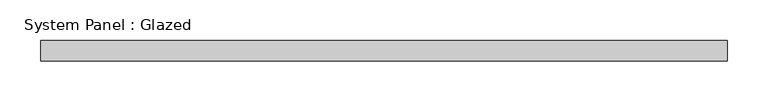
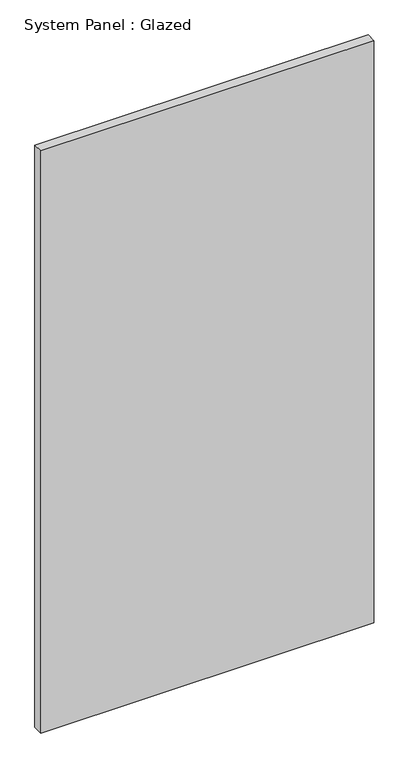
"""IFC4 building model written with IfcOpenShell, lengths in millimetres: plate geometry, System Panel : Glazed."""

from ifc_helpers import new_model, si_unit, origin, origin_with_axes, place, context, project, spatial, polyline, outline, extrude, source, transform, mapped, element, save


def system_panel_glazed_e66cc300(model_context):
    return source(origin(), model_context, "Body", "SweptSolid", [
        extrude(outline(polyline([(422.275, 19.05), (-422.275, 19.05), (-422.275, 44.45), (422.275, 44.45), (422.275, 19.05)])), origin_with_axes(), (0.0, 0.0, 1.0), 1559.8910355),
    ])


if __name__ == "__main__":
    model = new_model("IFC4")
    model_context = context("Model", 3, world=origin())
    ifc_project = project(units=[si_unit("LENGTHUNIT", "METRE", prefix="MILLI")], contexts=[model_context])
    site = spatial("IfcSite", under=ifc_project)
    building = spatial("IfcBuilding", under=site)
    placement = place(None, origin())
    system_panel_glazed_shape = system_panel_glazed_e66cc300(model_context)
    element("IfcPlate", 1, ObjectType="System Panel : Glazed", at=placement, inside=building, context=model_context, shape_type="MappedRepresentation", body=[
        mapped(system_panel_glazed_shape, transform((0.0, 0.0, 0.0), x_axis=(1.0, 0.0, 0.0), y_axis=(0.0, 1.0, 0.0), z_axis=(0.0, 0.0, 1.0))),
    ])
    save(model, "model.ifc")

# Revit data of these elements
# Type "System Panel : Glazed"
#   Construction Type Id = "GSP4R"
#   Analytic Construction = "1/8 in Pilkington single glazing"
#   Visual Light Transmittance = 0.9
#   Solar Heat Gain Coefficient = 0.86
#   Heat Transfer Coefficient (U) = 1.18115 BTU/(h·ft²·°F)
#   Define Thermal Properties by = 1
# Element 1 (IfcPlate, "System Panel : Glazed")
#   Materials on its faces: "Glass"
# Materials
#   "Glass": class "Glass", colour RGB 0 128 192, transparency 0.75, Description = "Soda Lime Glass", Cost = 0
